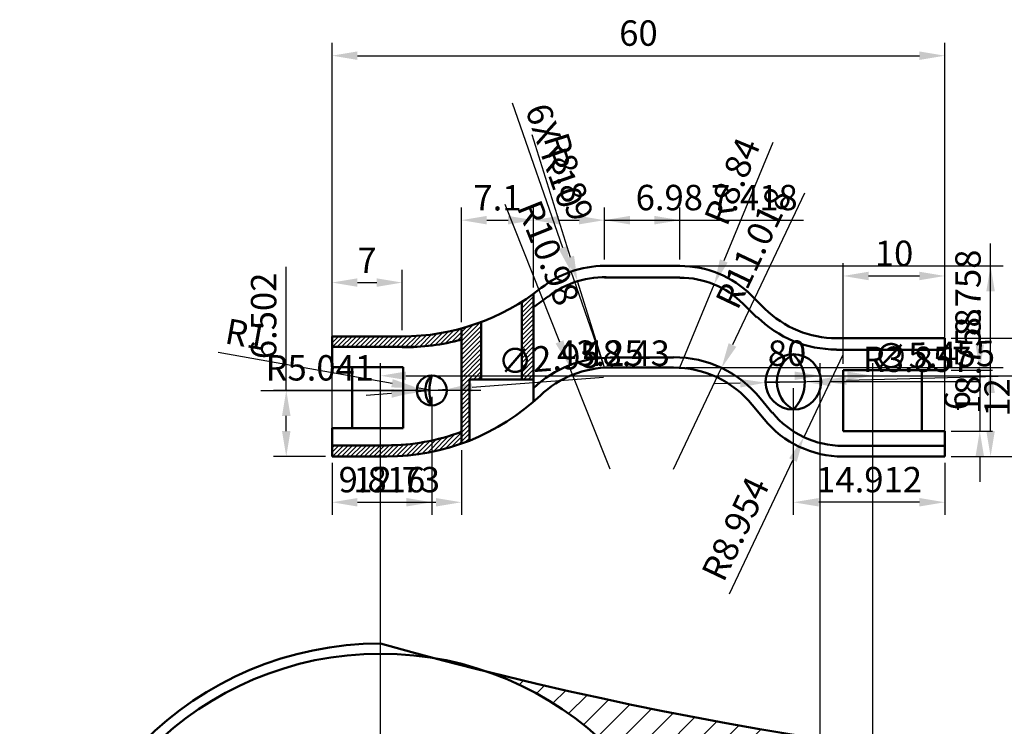
# Model space of a CAD drawing. Units: millimetres. Extents: x 1605 to 2079, y 1280 to 1879.
# Tile 3 of 7: x 1648 to 1745, y 1514 to 1583. Entities that reach past the tile are written whole.
import ezdxf

# ---------------------------------------------------------------- set-up
doc = ezdxf.new("R2010")
doc.units = ezdxf.units.MM
doc.linetypes.add('CENTER2', pattern=[28.574999999999996, 19.05, -3.174999999999999, 3.174999999999999, -3.174999999999999])
for name, color, linetype, lineweight in [('M-CNTR', 1, 'CENTER2', 18), ('M-DIMS', 2, 'Continuous', 25), ('M-HATC', 8, 'Continuous', 18), ('M-OUTL', 7, 'Continuous', 50)]:
    doc.layers.add(name, color=color, linetype=linetype, lineweight=lineweight)
doc.styles.get("Standard").update_dxf_attribs({"font": 'arial.ttf'})
doc.dimstyles.new('ISO-25', dxfattribs={"dimtxt": 2.5, "dimasz": 2.5, "dimexe": 1.25, "dimexo": 0.625, "dimtad": 1, "dimdec": 0, "dimtxsty": 'Standard', "dimcen": 2.5, "dimadec": 0, "dimazin": 0, "dimtfac": 1, "dimtdec": 0, "dimtmove": 0, "dimatfit": 3, "dimfxl": 1, "dimarcsym": 0})
pattern_1 = [(45, (0, 0), (-0.2245064030267288, 0.2245064030267288), [])]

# ---------------------------------------------------------------- blocks, each defined once
blk = doc.blocks.new('*U2')
at = {"layer": 'M-CNTR', "color": 0, "transparency": 16777216}
for p, q in [((0, 6.4), (0, 35.5)), ((-35.5, 0), (-6.399999999999998, 0)), ((6.4, 0), (35.5, 0)), ((0, -35.5), (0, -6.399999999999998))]:
    blk.add_line(p, q, dxfattribs=at)
at = {"layer": 'M-CNTR', "color": 0, "linetype": 'Continuous', "transparency": 16777216}
for p, q in [((0, -3.2), (0, 3.2)), ((-3.2, 0), (3.2, 0))]:
    blk.add_line(p, q, dxfattribs=at)
blk = doc.blocks.new('*D6')
at = {"layer": 'Defpoints', "color": 0, "transparency": 16777216}
for p in [(1738.945829042659, 1579.826881590476), (1678.645044474844, 1540.384347719754), (1738.945829042659, 1540.384347719754)]:
    blk.add_point(p, dxfattribs=at)
at = {"layer": 'M-DIMS', "color": 0, "lineweight": -2, "transparency": 16777216}
for p, q in [((1678.645044474844, 1541.009347719754), (1678.645044474844, 1581.076881590476)), ((1738.945829042659, 1541.009347719754), (1738.945829042659, 1581.076881590476)), ((1681.145044474844, 1579.826881590476), (1736.445829042659, 1579.826881590476))]:
    blk.add_line(p, q, dxfattribs=at)
at = {"layer": 'M-DIMS', "color": 0, "transparency": 16777216}
for points in [[(1681.145044474844, 1580.243548257142), (1681.145044474844, 1579.410214923809), (1678.645044474844, 1579.826881590476)], [(1736.445829042659, 1580.243548257142), (1736.445829042659, 1579.410214923809), (1738.945829042659, 1579.826881590476)]]:
    blk.add_solid(points, dxfattribs=at)
at = {"layer": 'M-DIMS', "color": 0, "transparency": 16777216, "insert": (1708.795436758752, 1581.72831405978), "char_height": 2.5, "attachment_point": 5}
blk.add_mtext('60', dxfattribs=at)
blk = doc.blocks.new('*D7')
at = {"layer": 'Defpoints', "color": 0, "transparency": 16777216}
for p in [(1685.55133154725, 1557.502449097515), (1678.645044474844, 1552.199565545558), (1685.55133154725, 1552.199565545558)]:
    blk.add_point(p, dxfattribs=at)
at = {"layer": 'M-DIMS', "color": 0, "lineweight": -2, "transparency": 16777216}
for p, q in [((1678.645044474844, 1552.824565545557), (1678.645044474844, 1558.752449097515)), ((1685.55133154725, 1552.824565545557), (1685.55133154725, 1558.752449097515)), ((1681.145044474844, 1557.502449097515), (1683.05133154725, 1557.502449097515))]:
    blk.add_line(p, q, dxfattribs=at)
at = {"layer": 'M-DIMS', "color": 0, "transparency": 16777216}
for points in [[(1681.145044474844, 1557.919115764181), (1681.145044474844, 1557.085782430848), (1678.645044474844, 1557.502449097515)], [(1683.05133154725, 1557.919115764181), (1683.05133154725, 1557.085782430848), (1685.55133154725, 1557.502449097515)]]:
    blk.add_solid(points, dxfattribs=at)
at = {"layer": 'M-DIMS', "color": 0, "transparency": 16777216, "insert": (1682.098188011047, 1559.377449097515), "char_height": 2.5, "attachment_point": 5}
blk.add_mtext('7', dxfattribs=at)
blk = doc.blocks.new('*D8')
at = {"layer": 'Defpoints', "color": 0, "transparency": 16777216}
for p in [(1738.94582904266, 1552.020572380303), (1738.94582904266, 1540.384347719755), (1746.290883843988, 1540.384347719755)]:
    blk.add_point(p, dxfattribs=at)
at = {"layer": 'M-DIMS', "color": 0, "lineweight": -2, "transparency": 16777216}
for p, q in [((1739.57082904266, 1552.020572380303), (1747.540883843988, 1552.020572380303)), ((1746.290883843988, 1549.520572380303), (1746.290883843988, 1542.884347719755)), ((1739.57082904266, 1540.384347719755), (1747.540883843988, 1540.384347719755))]:
    blk.add_line(p, q, dxfattribs=at)
at = {"layer": 'M-DIMS', "color": 0, "transparency": 16777216}
for points in [[(1745.874217177321, 1549.520572380303), (1746.707550510654, 1549.520572380303), (1746.290883843988, 1552.020572380303)], [(1745.874217177321, 1542.884347719755), (1746.707550510654, 1542.884347719755), (1746.290883843988, 1540.384347719755)]]:
    blk.add_solid(points, dxfattribs=at)
at = {"layer": 'M-DIMS', "color": 0, "transparency": 16777216, "insert": (1744.410767882187, 1546.202460050028), "char_height": 2.5, "attachment_point": 5, "rotation": 90}
blk.add_mtext('12', dxfattribs=at)
blk = doc.blocks.new('*D9')
at = {"layer": 'Defpoints', "color": 0, "transparency": 16777216}
for p in [(1738.94582904266, 1548.883072039406), (1738.94582904266, 1542.883072039406), (1742.3810871375, 1542.883072039406)]:
    blk.add_point(p, dxfattribs=at)
at = {"layer": 'M-DIMS', "color": 0, "lineweight": -2, "transparency": 16777216}
for p, q in [((1742.3810871375, 1551.383072039406), (1742.3810871375, 1553.883072039406)), ((1739.57082904266, 1548.883072039406), (1743.6310871375, 1548.883072039406)), ((1742.3810871375, 1548.883072039406), (1742.3810871375, 1542.883072039406)), ((1739.57082904266, 1542.883072039406), (1743.6310871375, 1542.883072039406)), ((1742.3810871375, 1540.383072039406), (1742.3810871375, 1537.883072039406))]:
    blk.add_line(p, q, dxfattribs=at)
at = {"layer": 'M-DIMS', "color": 0, "transparency": 16777216}
for points in [[(1741.964420470833, 1551.383072039406), (1742.797753804167, 1551.383072039406), (1742.3810871375, 1548.883072039406)], [(1741.964420470833, 1540.383072039406), (1742.797753804167, 1540.383072039406), (1742.3810871375, 1542.883072039406)]]:
    blk.add_solid(points, dxfattribs=at)
at = {"layer": 'M-DIMS', "color": 0, "transparency": 16777216, "insert": (1740.479654668195, 1545.883072039405), "char_height": 2.5, "attachment_point": 5, "rotation": 90}
blk.add_mtext('6', dxfattribs=at)
blk = doc.blocks.new('*D10')
at = {"layer": 'Defpoints', "color": 0, "transparency": 16777216}
for p in [(1738.945829042659, 1558.149744778363), (1728.945829042659, 1548.883072039405), (1738.945829042659, 1548.883072039405)]:
    blk.add_point(p, dxfattribs=at)
at = {"layer": 'M-DIMS', "color": 0, "lineweight": -2, "transparency": 16777216}
for p, q in [((1728.945829042659, 1549.508072039405), (1728.945829042659, 1559.399744778363)), ((1738.945829042659, 1549.508072039405), (1738.945829042659, 1559.399744778363)), ((1731.445829042659, 1558.149744778363), (1736.445829042659, 1558.149744778363))]:
    blk.add_line(p, q, dxfattribs=at)
at = {"layer": 'M-DIMS', "color": 0, "transparency": 16777216}
for points in [[(1731.445829042659, 1558.56641144503), (1731.445829042659, 1557.733078111696), (1728.945829042659, 1558.149744778363)], [(1736.445829042659, 1558.56641144503), (1736.445829042659, 1557.733078111696), (1738.945829042659, 1558.149744778363)]]:
    blk.add_solid(points, dxfattribs=at)
at = {"layer": 'M-DIMS', "color": 0, "transparency": 16777216, "insert": (1733.945829042659, 1560.051177247667), "char_height": 2.5, "attachment_point": 5}
blk.add_mtext('10', dxfattribs=at)
blk = doc.blocks.new('*D11')
at = {"layer": 'Defpoints', "color": 0, "transparency": 16777216}
for p in [(1687.009202827217, 1547.147898341788), (1688.460822472765, 1546.886649148962)]:
    blk.add_point(p, dxfattribs=at)
at = {"layer": 'M-DIMS', "color": 0, "lineweight": -2, "transparency": 16777216}
for p, q in [((1667.454793814781, 1550.667121566922), (1684.548732004864, 1547.590711318507)), ((1688.460822472765, 1546.886649148962), (1687.009202827217, 1547.147898341788))]:
    blk.add_line(p, q, dxfattribs=at)
at = {"layer": 'M-DIMS', "color": 0, "transparency": 16777216}
blk.add_solid([(1684.622534167651, 1548.000789788899), (1684.474929842078, 1547.180632848115), (1687.009202827217, 1547.147898341788)], dxfattribs=at)
at = {"layer": 'M-DIMS', "color": 0, "transparency": 16777216, "insert": (1670.149257494102, 1552.092518035817), "char_height": 2.5, "attachment_point": 5, "rotation": 349.79764513890115}
blk.add_mtext('R1', dxfattribs=at)
blk = doc.blocks.new('*D45')
at = {"layer": 'Defpoints', "color": 0, "transparency": 16777216}
for p in [(1763.415856, 1548.330601), (1683.415856, 1488.980601), (1763.415856, 1488.980601)]:
    blk.add_point(p, dxfattribs=at)
at = {"layer": 'M-DIMS', "color": 0, "lineweight": -2, "transparency": 16777216}
for p, q in [((1683.415856, 1489.605601), (1683.415856, 1549.580601)), ((1763.415856, 1489.605601), (1763.415856, 1549.580601)), ((1685.915856, 1548.330601), (1760.915856, 1548.330601))]:
    blk.add_line(p, q, dxfattribs=at)
at = {"layer": 'M-DIMS', "color": 0, "transparency": 16777216}
for points in [[(1685.915856, 1548.747267666666), (1685.915856, 1547.913934333333), (1683.415856, 1548.330601)], [(1760.915856, 1548.747267666666), (1760.915856, 1547.913934333333), (1763.415856, 1548.330601)]]:
    blk.add_solid(points, dxfattribs=at)
at = {"layer": 'M-DIMS', "color": 0, "transparency": 16777216, "insert": (1723.415856, 1550.232033469304), "char_height": 2.5, "attachment_point": 5}
blk.add_mtext('80', dxfattribs=at)
blk = doc.blocks.new('*D47')
at = {"layer": 'Defpoints', "color": 0, "transparency": 16777216}
for p in [(1726.666293, 1548.330601), (1683.415856, 1488.980601), (1726.666293, 1452.487829)]:
    blk.add_point(p, dxfattribs=at)
at = {"layer": 'M-DIMS', "color": 0, "lineweight": -2, "transparency": 16777216}
for p, q in [((1683.415856, 1489.605601), (1683.415856, 1549.580601)), ((1726.666293, 1453.112829), (1726.666293, 1549.580601)), ((1685.915856, 1548.330601), (1724.166293, 1548.330601))]:
    blk.add_line(p, q, dxfattribs=at)
at = {"layer": 'M-DIMS', "color": 0, "transparency": 16777216}
for points in [[(1685.915856, 1548.747267666666), (1685.915856, 1547.913934333333), (1683.415856, 1548.330601)], [(1724.166293, 1548.747267666666), (1724.166293, 1547.913934333333), (1726.666293, 1548.330601)]]:
    blk.add_solid(points, dxfattribs=at)
at = {"layer": 'M-DIMS', "color": 0, "transparency": 16777216, "insert": (1705.0410745, 1550.232886129604), "char_height": 2.5, "attachment_point": 5}
blk.add_mtext('43.25', dxfattribs=at)
blk = doc.blocks.new('*D49')
at = {"layer": 'Defpoints', "color": 0, "transparency": 16777216}
for p in [(1731.842463, 1548.330601), (1731.842463, 1511.839336), (1683.415856, 1488.980601)]:
    blk.add_point(p, dxfattribs=at)
at = {"layer": 'M-DIMS', "color": 0, "lineweight": -2, "transparency": 16777216}
for p, q in [((1683.415856, 1489.605601), (1683.415856, 1549.580601)), ((1731.842463, 1512.464336), (1731.842463, 1549.580601)), ((1685.915856, 1548.330601), (1729.342463, 1548.330601))]:
    blk.add_line(p, q, dxfattribs=at)
at = {"layer": 'M-DIMS', "color": 0, "transparency": 16777216}
for points in [[(1685.915856, 1548.747267666666), (1685.915856, 1547.913934333333), (1683.415856, 1548.330601)], [(1729.342463, 1548.747267666666), (1729.342463, 1547.913934333333), (1731.842463, 1548.330601)]]:
    blk.add_solid(points, dxfattribs=at)
at = {"layer": 'M-DIMS', "color": 0, "transparency": 16777216, "insert": (1707.6291595, 1550.232886129604), "char_height": 2.5, "attachment_point": 5}
blk.add_mtext('48.43', dxfattribs=at)
blk = doc.blocks.new('*D52')
at = {"layer": 'Defpoints', "color": 0, "transparency": 16777216}
for p in [(1712.872269000001, 1559.142254000001), (1743.445829000002, 1559.142254000001), (1738.945829000001, 1540.384348000001)]:
    blk.add_point(p, dxfattribs=at)
at = {"layer": 'M-DIMS', "color": 0, "lineweight": -2, "transparency": 16777216}
for p, q in [((1713.497269000001, 1559.142254000001), (1744.695829000002, 1559.142254000001)), ((1743.445829000002, 1542.884348000001), (1743.445829000002, 1556.642254000001)), ((1739.570829000001, 1540.384348000001), (1744.695829000002, 1540.384348000001))]:
    blk.add_line(p, q, dxfattribs=at)
at = {"layer": 'M-DIMS', "color": 0, "transparency": 16777216}
for points in [[(1743.029162333335, 1556.642254000001), (1743.862495666668, 1556.642254000001), (1743.445829000002, 1559.142254000001)], [(1743.029162333335, 1542.884348000001), (1743.862495666668, 1542.884348000001), (1743.445829000002, 1540.384348000001)]]:
    blk.add_solid(points, dxfattribs=at)
at = {"layer": 'M-DIMS', "color": 0, "transparency": 16777216, "insert": (1741.544396530698, 1549.763301), "char_height": 2.5, "attachment_point": 5, "rotation": 90}
blk.add_mtext('18.758', dxfattribs=at)
blk = doc.blocks.new('*D53')
at = {"layer": 'Defpoints', "color": 0, "transparency": 16777216}
for p in [(1691.374813, 1541.647874), (1678.645044, 1540.384348), (1691.374813, 1535.884348)]:
    blk.add_point(p, dxfattribs=at)
at = {"layer": 'M-DIMS', "color": 0, "lineweight": -2, "transparency": 16777216}
for p, q in [((1691.374813, 1541.022874), (1691.374813, 1534.634348)), ((1678.645044, 1539.759348), (1678.645044, 1534.634348)), ((1681.145044, 1535.884348), (1688.874813, 1535.884348))]:
    blk.add_line(p, q, dxfattribs=at)
at = {"layer": 'M-DIMS', "color": 0, "transparency": 16777216}
for points in [[(1681.145044, 1536.301014666667), (1681.145044, 1535.467681333333), (1678.645044, 1535.884348)], [(1688.874813, 1536.301014666667), (1688.874813, 1535.467681333333), (1691.374813, 1535.884348)]]:
    blk.add_solid(points, dxfattribs=at)
at = {"layer": 'M-DIMS', "color": 0, "transparency": 16777216, "insert": (1685.0099285, 1537.786633129604), "char_height": 2.5, "attachment_point": 5}
blk.add_mtext('12.73', dxfattribs=at)
blk = doc.blocks.new('*D54')
at = {"layer": 'Defpoints', "color": 0, "transparency": 16777216}
for p in [(1698.474129, 1563.642254), (1698.474129, 1556.395035), (1691.374813, 1552.98431)]:
    blk.add_point(p, dxfattribs=at)
at = {"layer": 'M-DIMS', "color": 0, "lineweight": -2, "transparency": 16777216}
for p, q in [((1691.374813, 1553.60931), (1691.374813, 1564.892254)), ((1698.474129, 1557.020035), (1698.474129, 1564.892254)), ((1693.874813, 1563.642254), (1695.974129, 1563.642254))]:
    blk.add_line(p, q, dxfattribs=at)
at = {"layer": 'M-DIMS', "color": 0, "transparency": 16777216}
for points in [[(1693.874813, 1564.058920666667), (1693.874813, 1563.225587333333), (1691.374813, 1563.642254)], [(1695.974129, 1564.058920666667), (1695.974129, 1563.225587333333), (1698.474129, 1563.642254)]]:
    blk.add_solid(points, dxfattribs=at)
at = {"layer": 'M-DIMS', "color": 0, "transparency": 16777216, "insert": (1694.924471, 1565.522369961801), "char_height": 2.5, "attachment_point": 5}
blk.add_mtext('7.1', dxfattribs=at)
blk = doc.blocks.new('*D55')
at = {"layer": 'Defpoints', "color": 0, "transparency": 16777216}
for p in [(1705.454375, 1563.642254), (1705.454375, 1559.142254), (1698.474129, 1556.395035)]:
    blk.add_point(p, dxfattribs=at)
at = {"layer": 'M-DIMS', "color": 0, "lineweight": -2, "transparency": 16777216}
for p, q in [((1698.474129, 1557.020035), (1698.474129, 1564.892254)), ((1705.454375, 1559.767254), (1705.454375, 1564.892254)), ((1700.974129, 1563.642254), (1702.954375, 1563.642254)), ((1705.454375, 1563.642254), (1715.716994372442, 1563.642254))]:
    blk.add_line(p, q, dxfattribs=at)
at = {"layer": 'M-DIMS', "color": 0, "transparency": 16777216}
for points in [[(1700.974129, 1564.058920666667), (1700.974129, 1563.225587333333), (1698.474129, 1563.642254)], [(1702.954375, 1564.058920666667), (1702.954375, 1563.225587333333), (1705.454375, 1563.642254)]]:
    blk.add_solid(points, dxfattribs=at)
at = {"layer": 'M-DIMS', "color": 0, "transparency": 16777216, "insert": (1711.835684686221, 1565.543686469304), "char_height": 2.5, "attachment_point": 5}
blk.add_mtext('6.98', dxfattribs=at)
blk = doc.blocks.new('*D56')
at = {"layer": 'Defpoints', "color": 0, "transparency": 16777216}
for p in [(1712.872269, 1563.642254), (1705.454375, 1559.142254), (1712.872269, 1559.142254)]:
    blk.add_point(p, dxfattribs=at)
at = {"layer": 'M-DIMS', "color": 0, "lineweight": -2, "transparency": 16777216}
for p, q in [((1705.454375, 1559.767254), (1705.454375, 1564.892254)), ((1712.872269, 1559.767254), (1712.872269, 1564.892254)), ((1707.954375, 1563.642254), (1710.372269, 1563.642254)), ((1712.872269, 1563.642254), (1725.043142124147, 1563.642254))]:
    blk.add_line(p, q, dxfattribs=at)
at = {"layer": 'M-DIMS', "color": 0, "transparency": 16777216}
for points in [[(1707.954375, 1564.058920666667), (1707.954375, 1563.225587333333), (1705.454375, 1563.642254)], [(1710.372269, 1564.058920666667), (1710.372269, 1563.225587333333), (1712.872269, 1563.642254)]]:
    blk.add_solid(points, dxfattribs=at)
at = {"layer": 'M-DIMS', "color": 0, "transparency": 16777216, "insert": (1720.207705562074, 1565.543686469304), "char_height": 2.5, "attachment_point": 5}
blk.add_mtext('7.418', dxfattribs=at)
blk = doc.blocks.new('*D57')
at = {"layer": 'Defpoints', "color": 0, "transparency": 16777216}
for p in [(1688.460822, 1546.886649), (1678.645044, 1540.384348), (1688.460822, 1535.884348)]:
    blk.add_point(p, dxfattribs=at)
at = {"layer": 'M-DIMS', "color": 0, "lineweight": -2, "transparency": 16777216}
for p, q in [((1688.460822, 1546.261649), (1688.460822, 1534.634348)), ((1678.645044, 1539.759348), (1678.645044, 1534.634348)), ((1681.145044, 1535.884348), (1685.960822, 1535.884348))]:
    blk.add_line(p, q, dxfattribs=at)
at = {"layer": 'M-DIMS', "color": 0, "transparency": 16777216}
for points in [[(1681.145044, 1536.301014666667), (1681.145044, 1535.467681333333), (1678.645044, 1535.884348)], [(1685.960822, 1536.301014666667), (1685.960822, 1535.467681333333), (1688.460822, 1535.884348)]]:
    blk.add_solid(points, dxfattribs=at)
at = {"layer": 'M-DIMS', "color": 0, "transparency": 16777216, "insert": (1683.552933, 1537.785780469304), "char_height": 2.5, "attachment_point": 5}
blk.add_mtext('9.816', dxfattribs=at)
blk = doc.blocks.new('*D58')
at = {"layer": 'Defpoints', "color": 0, "transparency": 16777216}
for p in [(1674.145044000002, 1546.886649000001), (1688.460822000001, 1546.886649000001), (1678.645044000001, 1540.384348000001)]:
    blk.add_point(p, dxfattribs=at)
at = {"layer": 'M-DIMS', "color": 0, "lineweight": -2, "transparency": 16777216}
for p, q in [((1674.145044000002, 1546.886649000001), (1674.145044000002, 1559.060932765349)), ((1687.835822000001, 1546.886649000001), (1672.895044000002, 1546.886649000001)), ((1674.145044000002, 1542.884348000001), (1674.145044000002, 1544.386649000001)), ((1678.020044000001, 1540.384348000001), (1672.895044000002, 1540.384348000001))]:
    blk.add_line(p, q, dxfattribs=at)
at = {"layer": 'M-DIMS', "color": 0, "transparency": 16777216}
for points in [[(1673.728377333335, 1544.386649000001), (1674.561710666668, 1544.386649000001), (1674.145044000002, 1546.886649000001)], [(1673.728377333335, 1542.884348000001), (1674.561710666668, 1542.884348000001), (1674.145044000002, 1540.384348000001)]]:
    blk.add_solid(points, dxfattribs=at)
at = {"layer": 'M-DIMS', "color": 0, "transparency": 16777216, "insert": (1672.243611530698, 1554.223790882674), "char_height": 2.5, "attachment_point": 5, "rotation": 90}
blk.add_mtext('6.502', dxfattribs=at)
blk = doc.blocks.new('*D59')
at = {"layer": 'Defpoints', "color": 0, "transparency": 16777216}
for p in [(1724.033427, 1547.729634), (1738.945829, 1540.384348), (1724.033427, 1535.884348)]:
    blk.add_point(p, dxfattribs=at)
at = {"layer": 'M-DIMS', "color": 0, "lineweight": -2, "transparency": 16777216}
for p, q in [((1724.033427, 1547.104634), (1724.033427, 1534.634348)), ((1738.945829, 1539.759348), (1738.945829, 1534.634348)), ((1736.445829, 1535.884348), (1726.533427, 1535.884348))]:
    blk.add_line(p, q, dxfattribs=at)
at = {"layer": 'M-DIMS', "color": 0, "transparency": 16777216}
for points in [[(1726.533427, 1536.301014666667), (1726.533427, 1535.467681333333), (1724.033427, 1535.884348)], [(1736.445829, 1536.301014666667), (1736.445829, 1535.467681333333), (1738.945829, 1535.884348)]]:
    blk.add_solid(points, dxfattribs=at)
at = {"layer": 'M-DIMS', "color": 0, "transparency": 16777216, "insert": (1731.489628, 1537.785780469304), "char_height": 2.5, "attachment_point": 5}
blk.add_mtext('14.912', dxfattribs=at)
blk = doc.blocks.new('*D60')
at = {"layer": 'Defpoints', "color": 0, "transparency": 16777216}
for p in [(1712.872269000001, 1549.142254000001), (1743.445829000002, 1549.142254000001), (1738.945829000001, 1540.384348000001)]:
    blk.add_point(p, dxfattribs=at)
at = {"layer": 'M-DIMS', "color": 0, "lineweight": -2, "transparency": 16777216}
for p, q in [((1743.445829000002, 1549.142254000001), (1743.445829000002, 1561.337001612552)), ((1713.497269000001, 1549.142254000001), (1744.695829000002, 1549.142254000001)), ((1743.445829000002, 1542.884348000001), (1743.445829000002, 1546.642254000001)), ((1739.570829000001, 1540.384348000001), (1744.695829000002, 1540.384348000001))]:
    blk.add_line(p, q, dxfattribs=at)
at = {"layer": 'M-DIMS', "color": 0, "transparency": 16777216}
for points in [[(1743.029162333335, 1546.642254000001), (1743.862495666668, 1546.642254000001), (1743.445829000002, 1549.142254000001)], [(1743.029162333335, 1542.884348000001), (1743.862495666668, 1542.884348000001), (1743.445829000002, 1540.384348000001)]]:
    blk.add_solid(points, dxfattribs=at)
at = {"layer": 'M-DIMS', "color": 0, "transparency": 16777216, "insert": (1741.544396530698, 1556.489627806275), "char_height": 2.5, "attachment_point": 5, "rotation": 90}
blk.add_mtext('8.758', dxfattribs=at)
blk = doc.blocks.new('*D73')
at = {"layer": 'Defpoints', "color": 0, "transparency": 16777216}
for p in [(1702.160883, 1558.584336), (1705.454374999999, 1549.142254)]:
    blk.add_point(p, dxfattribs=at)
at = {"layer": 'M-DIMS', "color": 0, "lineweight": -2, "transparency": 16777216}
for p, q in [((1696.36413494683, 1575.202979813729), (1701.337510008434, 1560.944856475819)), ((1705.454374999999, 1549.142254), (1702.160883, 1558.584336))]:
    blk.add_line(p, q, dxfattribs=at)
at = {"layer": 'M-DIMS', "color": 0, "transparency": 16777216}
blk.add_solid([(1701.730930087737, 1561.082085307746), (1700.944089929131, 1560.807627643891), (1702.160883, 1558.584336)], dxfattribs=at)
at = {"layer": 'M-DIMS', "color": 0, "transparency": 16777216, "insert": (1700.234484092722, 1569.880413638887), "char_height": 2.5, "attachment_point": 5, "rotation": 289.22927914580976}
blk.add_mtext('6X R10', dxfattribs=at)
blk = doc.blocks.new('*D74')
at = {"layer": 'Defpoints', "color": 0, "transparency": 16777216}
for p in [(1716.975232, 1549.099488999999), (1712.257654, 1539.142253999999)]:
    blk.add_point(p, dxfattribs=at)
at = {"layer": 'M-DIMS', "color": 0, "lineweight": -2, "transparency": 16777216}
for p, q in [((1725.12151537231, 1566.293578406614), (1718.045631876652, 1551.358746423151)), ((1712.257654, 1539.142253999999), (1716.975232, 1549.099488999999))]:
    blk.add_line(p, q, dxfattribs=at)
at = {"layer": 'M-DIMS', "color": 0, "transparency": 16777216}
blk.add_solid([(1717.669088972794, 1551.537146402593), (1718.422174780511, 1551.180346443709), (1716.975232, 1549.099488999999)], dxfattribs=at)
at = {"layer": 'M-DIMS', "color": 0, "transparency": 16777216, "insert": (1720.400443394449, 1560.7699083587), "char_height": 2.5, "attachment_point": 5, "rotation": 64.64915745028115}
blk.add_mtext('R11.018', dxfattribs=at)
blk = doc.blocks.new('*D75')
at = {"layer": 'Defpoints', "color": 0, "transparency": 16777216}
for p in [(1701.959906999999, 1549.344234999999), (1706.022004999999, 1539.142254)]:
    blk.add_point(p, dxfattribs=at)
at = {"layer": 'M-DIMS', "color": 0, "lineweight": -2, "transparency": 16777216}
for p, q in [((1695.640185789668, 1565.21624884927), (1701.035100522225, 1551.666891448695)), ((1706.022004999999, 1539.142254), (1701.959906999999, 1549.344234999999))]:
    blk.add_line(p, q, dxfattribs=at)
at = {"layer": 'M-DIMS', "color": 0, "transparency": 16777216}
blk.add_solid([(1701.42220993034, 1551.821025861657), (1700.647991114109, 1551.512757035732), (1701.959906999999, 1549.344234999999)], dxfattribs=at)
at = {"layer": 'M-DIMS', "color": 0, "transparency": 16777216, "insert": (1699.641789671695, 1560.306281199195), "char_height": 2.5, "attachment_point": 5, "rotation": 291.71084335696685}
blk.add_mtext('R10.98', dxfattribs=at)
blk = doc.blocks.new('*D76')
at = {"layer": 'Defpoints', "color": 0, "transparency": 16777216}
for p in [(1728.901096, 1550.384348), (1725.067011, 1542.293023)]:
    blk.add_point(p, dxfattribs=at)
at = {"layer": 'M-DIMS', "color": 0, "lineweight": -2, "transparency": 16777216}
for p, q in [((1728.901096, 1550.384348), (1725.067011, 1542.293023)), ((1717.758091055393, 1526.868522324926), (1723.996486807893, 1540.033824479702))]:
    blk.add_line(p, q, dxfattribs=at)
at = {"layer": 'M-DIMS', "color": 0, "transparency": 16777216}
blk.add_solid([(1723.619953721177, 1540.212245178387), (1724.373019894609, 1539.855403781018), (1725.067011, 1542.293023)], dxfattribs=at)
at = {"layer": 'M-DIMS', "color": 0, "transparency": 16777216, "insert": (1718.623741467151, 1533.135785925383), "char_height": 2.5, "attachment_point": 5, "rotation": 64.64600471361501}
blk.add_mtext('R8.954', dxfattribs=at)
blk = doc.blocks.new('*D77')
at = {"layer": 'Defpoints', "color": 0, "transparency": 16777216}
for p in [(1702.806965, 1557.629112999999), (1705.454374999999, 1549.142253999999)]:
    blk.add_point(p, dxfattribs=at)
at = {"layer": 'M-DIMS', "color": 0, "lineweight": -2, "transparency": 16777216}
for p, q in [((1698.297966980106, 1572.083704629602), (1702.062490273435, 1560.015691593196)), ((1705.454374999999, 1549.142253999999), (1702.806965, 1557.629112999999))]:
    blk.add_line(p, q, dxfattribs=at)
at = {"layer": 'M-DIMS', "color": 0, "transparency": 16777216}
blk.add_solid([(1702.460253372301, 1560.13977071429), (1701.664727174569, 1559.891612472102), (1702.806965, 1557.629112999999)], dxfattribs=at)
at = {"layer": 'M-DIMS', "color": 0, "transparency": 16777216, "insert": (1701.623158474549, 1567.809214775064), "char_height": 2.5, "attachment_point": 5, "rotation": 287.32490708382795}
blk.add_mtext('R8.89', dxfattribs=at)
blk = doc.blocks.new('*D78')
at = {"layer": 'Defpoints', "color": 0, "transparency": 16777216}
for p in [(1716.242073, 1557.315176), (1712.872269, 1549.142254)]:
    blk.add_point(p, dxfattribs=at)
at = {"layer": 'M-DIMS', "color": 0, "lineweight": -2, "transparency": 16777216}
for p, q in [((1722.007926505024, 1571.299333820451), (1717.195031425971, 1559.62642463188)), ((1712.872269, 1549.142254), (1716.242073, 1557.315176))]:
    blk.add_line(p, q, dxfattribs=at)
at = {"layer": 'M-DIMS', "color": 0, "transparency": 16777216}
blk.add_solid([(1716.809823320658, 1559.785251036209), (1717.580239531285, 1559.467598227552), (1716.242073, 1557.315176)], dxfattribs=at)
at = {"layer": 'M-DIMS', "color": 0, "transparency": 16777216, "insert": (1718.320084901166, 1567.343297979322), "char_height": 2.5, "attachment_point": 5, "rotation": 67.59299737995454}
blk.add_mtext('R8.84', dxfattribs=at)
blk = doc.blocks.new('*D79')
at = {"layer": 'Defpoints', "color": 0, "transparency": 16777216}
for p in [(1688.240238, 1546.887), (1693.281636, 1546.886649)]:
    blk.add_point(p, dxfattribs=at)
at = {"layer": 'M-DIMS', "color": 0, "lineweight": -2, "transparency": 16777216}
for p, q in [((1671.64405795837, 1546.888155484886), (1685.74023800606, 1546.887174058862)), ((1693.281636, 1546.886649), (1688.240238, 1546.887))]:
    blk.add_line(p, q, dxfattribs=at)
at = {"layer": 'M-DIMS', "color": 0, "transparency": 16777216}
blk.add_solid([(1685.74026701587, 1547.303840724518), (1685.740208996249, 1546.470507393205), (1688.240238, 1546.887)], dxfattribs=at)
at = {"layer": 'M-DIMS', "color": 0, "transparency": 16777216, "insert": (1677.442280369713, 1548.789184266), "char_height": 2.5, "attachment_point": 5, "rotation": 359.9960108647301}
blk.add_mtext('R5.041', dxfattribs=at)
blk = doc.blocks.new('*D80')
at = {"layer": 'Defpoints', "color": 0, "transparency": 16777216}
for p in [(1721.305945999999, 1547.729633999999), (1725.163186999999, 1547.729999999999)]:
    blk.add_point(p, dxfattribs=at)
at = {"layer": 'M-DIMS', "color": 0, "lineweight": -2, "transparency": 16777216}
for p, q in [((1721.305945999999, 1547.729633999999), (1725.163186999999, 1547.729999999999)), ((1742.241972734849, 1547.731620545767), (1727.663186988745, 1547.730237216185))]:
    blk.add_line(p, q, dxfattribs=at)
at = {"layer": 'M-DIMS', "color": 0, "transparency": 16777216}
blk.add_solid([(1727.663147452714, 1548.146903880976), (1727.663226524776, 1547.313570551394), (1725.163186999999, 1547.729999999999)], dxfattribs=at)
at = {"layer": 'M-DIMS', "color": 0, "transparency": 16777216, "insert": (1736.202399355041, 1549.63333261011), "char_height": 2.5, "attachment_point": 5, "rotation": 0.0054365945083347765}
blk.add_mtext('R3.857', dxfattribs=at)
blk = doc.blocks.new('*D81')
at = {"layer": 'Defpoints', "color": 0, "transparency": 16777216}
for p in [(1686.990023, 1546.776181), (1689.931621, 1546.997117)]:
    blk.add_point(p, dxfattribs=at)
at = {"layer": 'M-DIMS', "color": 0, "lineweight": -2, "transparency": 16777216}
for p, q in [((1705.370740907403, 1548.156710321676), (1692.424599277812, 1547.184358305163)), ((1684.497044722188, 1546.588939694837), (1682.004066444377, 1546.401698389674)), ((1686.990023, 1546.776181), (1689.931621, 1546.997117))]:
    blk.add_line(p, q, dxfattribs=at)
at = {"layer": 'M-DIMS', "color": 0, "transparency": 16777216}
for points in [[(1692.393392393618, 1547.599854684798), (1692.455806162006, 1546.768861925527), (1689.931621, 1546.997117)], [(1684.465837837994, 1547.004436074472), (1684.528251606382, 1546.173443315202), (1686.990023, 1546.776181)]]:
    blk.add_solid(points, dxfattribs=at)
at = {"layer": 'M-DIMS', "color": 0, "transparency": 16777216, "insert": (1699.996511926759, 1549.729968669378), "char_height": 2.5, "attachment_point": 5, "rotation": 4.295276733366178}
blk.add_mtext('∅2.95', dxfattribs=at)
blk = doc.blocks.new('*D82')
at = {"layer": 'Defpoints', "color": 0, "transparency": 16777216}
for p in [(1721.306873, 1547.658486), (1726.759981, 1547.800782)]:
    blk.add_point(p, dxfattribs=at)
at = {"layer": 'M-DIMS', "color": 0, "lineweight": -2, "transparency": 16777216}
for p, q in [((1744.179017402703, 1548.255322640669), (1729.259130282283, 1547.865995992877)), ((1718.807723717718, 1547.593272007122), (1716.308574435435, 1547.528058014245)), ((1721.306873, 1547.658486), (1726.759981, 1547.800782))]:
    blk.add_line(p, q, dxfattribs=at)
at = {"layer": 'M-DIMS', "color": 0, "transparency": 16777216}
for points in [[(1729.248261283469, 1548.282520873258), (1729.269999281095, 1547.449471112497), (1726.759981, 1547.800782)], [(1718.796854718904, 1548.009796887503), (1718.81859271653, 1547.176747126742), (1721.306873, 1547.658486)]]:
    blk.add_solid(points, dxfattribs=at)
at = {"layer": 'M-DIMS', "color": 0, "transparency": 16777216, "insert": (1737.917224625676, 1550.06394610197), "char_height": 2.5, "attachment_point": 5, "rotation": 1.494764176324067}
blk.add_mtext('∅5.455', dxfattribs=at)

msp = doc.modelspace()

# ---------------------------------------------------------------- hatches: boundary and pattern name
at = {"layer": 'M-HATC'}
h = msp.add_hatch(dxfattribs=at)
h.set_pattern_fill('ANSI31', color=256, scale=0.1)
h.set_pattern_definition(pattern_1)
h.paths.add_polyline_path([(1698.474128719783, 1556.395034851446, -0.0158606141869828), (1697.319423953205, 1555.611612427344), (1697.319423953205, 1547.976652959475), (1698.474128719783, 1547.976652959475)])
h = msp.add_hatch(dxfattribs=at)
h.set_pattern_fill('ANSI31', color=256, scale=0.1)
h.set_pattern_definition(pattern_1)
h.paths.add_polyline_path([(1693.319423953205, 1553.616642031816, -0.0232493374510837), (1691.374812892836, 1552.984310067067), (1691.374812892836, 1541.647873975909, 0.0095909802093284), (1692.164719186626, 1541.944965840922), (1692.164719186626, 1547.976652959475), (1693.319423953205, 1547.976652959475)])
h.paths.add_polyline_path([(1691.374812892836, 1541.647873975909), (1691.374812892836, 1542.817802922434, -0.0900572933523556), (1684.026435067029, 1541.483430706945), (1678.645044474844, 1541.483430706945), (1678.645044474844, 1540.384347719754), (1684.026435067029, 1540.384347719754, 0.0853469052335504)])
h.paths.add_polyline_path([(1691.374812892836, 1551.877660089471), (1691.374812892836, 1552.984310067067, -0.0670744800772869), (1685.551331547249, 1552.199565545558), (1678.645044474844, 1552.199565545558), (1678.645044474844, 1551.171994767597), (1686.933859029395, 1551.171994767597, 0.0488468451239397)])
h = msp.add_hatch(dxfattribs=at)
h.set_pattern_fill('ANSI31', color=256, scale=0.5700000000000001)
h.set_pattern_definition([(45, (0, 0), (-1.279686497252354, 1.279686497252354), [])])
edge = h.paths.add_edge_path()
edge.add_spline(control_points=[(1735.07459974606, 1431.314795075923), (1745.983278041014, 1442.572726331581), (1760.24984788448, 1457.296055612093), (1736.483989804082, 1465.949384402775), (1733.184296285201, 1487.573131299177), (1732.318614147286, 1503.228440483471), (1731.842462696298, 1511.83933570387)], knot_values=[0, 0, 0, 0, 32.3106591245444, 42.25647348148218, 64.0151754338639, 90.61240603446909, 90.61240603446909, 90.61240603446909, 90.61240603446909], degree=3, periodic=0)
edge.add_arc((1783.415855978972, 1878.806874192082), 370.5738647001252, 256.0328658121666, 262.00008128327465, ccw=False)
edge.add_arc((1683.415855978972, 1488.98060105796), 32, 0, 70.73817384477002, ccw=False)
edge.add_arc((1683.415855978972, 1488.98060105796), 32, -90, 0, ccw=False)
edge.add_line((1683.415855978972, 1456.98060105796), (1683.415855978972, 1455.98060105796))
edge.add_line((1683.415855978972, 1455.98060105796), (1735.07459974606, 1431.314795075923))
h.paths.add_polyline_path([(1726.66629323774, 1456.237829432783), (1741.66629323774, 1456.237829432783, -1), (1741.66629323774, 1448.737829432783), (1726.66629323774, 1448.737829432783, -1)], flags=16)
h.paths.add_polyline_path([(1731.47870797171, 1442.133012605171), (1736.613428299132, 1442.133012605171), (1736.613428299132, 1447.284786138595), (1731.47870797171, 1447.284786138595)], flags=24)
h.paths.add_polyline_path([(1713.173444990596, 1457.268825178529), (1718.453947385105, 1455.084302360538), (1720.423342620304, 1459.844791090414), (1715.142840225795, 1462.029313908404)], flags=24)

# ---------------------------------------------------------------- linework, layer by layer
at = {"layer": 'M-OUTL'}
for p, q in [((1705.454375346341, 1559.142254286537), (1712.872268745755, 1559.142254286537)), ((1705.454375346341, 1558.012835433478), (1712.872268745755, 1558.012835433478)), ((1698.474128719783, 1547.117880511772), (1698.474128719783, 1556.395034851446)), ((1719.920675000811, 1556.23591126046), (1721.238074599122, 1554.926915406378)), ((1697.319423953205, 1555.611612427344), (1697.319423953205, 1547.976652959475)), ((1719.090085348781, 1555.399989228672), (1720.407484947091, 1554.09099337459)), ((1691.374812892836, 1552.984310067067), (1691.374812892836, 1541.647873975909)), ((1693.319423953205, 1547.976652959475), (1693.319423953205, 1553.616642031816)), ((1678.645044474844, 1552.199565545558), (1685.55133154725, 1552.199565545558)), ((1678.645044474844, 1552.199565545558), (1678.645044474844, 1551.171994767597)), ((1728.286480854178, 1552.020572380302), (1738.945829042659, 1552.020572380302)), ((1738.945829042659, 1552.020572380302), (1738.945829042659, 1550.883072039405)), ((1678.645044474844, 1551.171994767597), (1686.933859029396, 1551.171994767597)), ((1678.645044474844, 1551.171994767597), (1678.645044474844, 1549.171994767597)), ((1706.022004912832, 1550.134855091574), (1712.25765375976, 1550.134855091574)), ((1728.286480854178, 1550.883072039405), (1738.945829042659, 1550.883072039405)), ((1738.945829042659, 1550.883072039405), (1738.945829042659, 1548.883072039405)), ((1678.645044474844, 1549.171994767597), (1685.645044474844, 1549.171994767597)), ((1680.636614060281, 1549.171994767597), (1680.63661406028, 1543.171994767597)), ((1685.645044474844, 1549.171994767597), (1685.645044474844, 1545.171994767597)), ((1706.022004912832, 1549.142254286536), (1712.25765375976, 1549.142254286536)), ((1738.945829042659, 1548.883072039405), (1728.945829042659, 1548.883072039405)), ((1728.945829042659, 1548.883072039405), (1728.945829042659, 1544.883072039405)), ((1736.680516214728, 1548.883072039405), (1736.680516214728, 1542.883072039405)), ((1692.164719186626, 1541.944965840922), (1692.164719186626, 1547.976652959475)), ((1692.164719186626, 1547.976652959475), (1698.474128719783, 1547.976652959475)), ((1695.319423953205, 1547.976652959475), (1693.319423953205, 1547.976652959475)), ((1698.474128719783, 1547.117880511772), (1698.474128719783, 1545.793261314212)), ((1719.996428487772, 1545.475607719678), (1721.162321112162, 1544.050994286612)), ((1720.784437397952, 1546.120508122138), (1721.950330022343, 1544.695894689072)), ((1685.645044474844, 1545.171994767597), (1685.645044474844, 1544.171994767597)), ((1728.945829042659, 1544.883072039405), (1728.945829042659, 1542.883072039405)), ((1685.645044474844, 1544.171994767597), (1685.645044474844, 1543.171994767597)), ((1681.645044474844, 1543.171994767597), (1678.645044474844, 1543.171994767597)), ((1678.645044474844, 1543.171994767597), (1678.645044474844, 1541.483430706945)), ((1685.645044474844, 1543.171994767597), (1681.645044474844, 1543.171994767597)), ((1728.945829042659, 1542.883072039405), (1738.945829042659, 1542.883072039405)), ((1738.945829042659, 1542.883072039405), (1738.945829042659, 1541.441282449549)), ((1678.645044474844, 1541.483430706945), (1684.026435067029, 1541.483430706945)), ((1678.645044474844, 1541.483430706945), (1678.645044474844, 1540.384347719754)), ((1728.901095840173, 1541.441282449549), (1738.945829042659, 1541.441282449549)), ((1738.945829042659, 1541.441282449549), (1738.945829042659, 1540.384347719754)), ((1678.645044474844, 1540.384347719754), (1684.026435067029, 1540.384347719754)), ((1728.901095840173, 1540.384347719754), (1738.945829042659, 1540.384347719754))]:
    msp.add_line(p, q, dxfattribs=at)
for centre, radius in [((1724.033427437432, 1547.729633627987), 2.727481313842424), ((1688.460822472767, 1546.886649148965), 1.474940926307681), ((1683.415855978972, 1488.98060105796), 32)]:
    msp.add_circle(centre, radius, dxfattribs=at)
for centre, radius, start, end in [((1705.454375346341, 1549.142254286537), 10, 90, 128.4601461444616), ((1712.872268745755, 1549.142254286536), 10, 45.18333013514169, 90), ((1705.454375346341, 1549.142254286537), 8.890193827309176, 86.19346029287718, 128.4601461444616), ((1712.872268745755, 1549.142254286536), 8.840375060270613, 45.18333013514169, 90), ((1685.55133154725, 1574.199565545557), 22, 270, 308.460146144462), ((1685.55133154725, 1574.199565545557), 23.06903548423432, 304.0682015065403, 308.460146144462), ((1728.286480854178, 1562.020572380302), 10, 225.1833301351417, 270), ((1728.286480854178, 1562.020572380302), 11.1079010127712, 225.1833301351417, 270), ((1685.55133154725, 1574.199565545557), 23.06903548423432, 270, 284.621776583433), ((1706.022004912832, 1539.142254286537), 10.98094024709417, 90, 133.4216144763459), ((1712.25765375976, 1539.142254286536), 11.01826056175077, 39.29662905253368, 90), ((1725.523062650189, 1547.729633627987), 3.10775922240486, 118.6415050293552, 241.3584949706419), ((1721.30594612359, 1547.729633627987), 3.857241065154974, 314.9999999999952, 45), ((1706.022004912832, 1539.142254286537), 10, 90, 133.4216144763459), ((1712.25765375976, 1539.142254286536), 10, 39.29662905253368, 90), ((1689.831735590376, 1546.886649148965), 2.013666683473275, 132.9065329178466, 227.0934670821507), ((1693.281636018545, 1546.886649148965), 5.041398018332984, 162.9883673170949, 197.0116326829047), ((1684.026435067029, 1562.384347719754), 22, 270, 313.4216144763454), ((1728.901095840173, 1550.384347719754), 8.953755626304364, 219.2966290525345, 270), ((1728.901095840173, 1550.384347719754), 10, 219.2966290525345, 270), ((1684.026435067029, 1562.384347719754), 20.90091701280926, 270, 290.5840833301981), ((1683.415855978972, 1488.98060105796), 33, 90, 270), ((1783.415855978972, 1878.806874192082), 370.5738647001254, 254.3445556403036, 285.6554443596963)]:
    msp.add_arc(centre, radius, start, end, dxfattribs=at)

# ---------------------------------------------------------------- block references
at = {"layer": 'M-CNTR'}
msp.add_blockref('*U2', (1683.415855978972, 1488.98060105796), dxfattribs=at)

# ---------------------------------------------------------------- dimensions: what is measured, and where the dimension line sits
at = {"layer": 'M-DIMS'}
for base, p1, p2, override, picture, middle in [((1738.945829042659, 1579.826881590476), (1678.645044474844, 1540.384347719754), (1738.945829042659, 1540.384347719754), {"dimclrd": 0, "dimclre": 0, "dimclrt": 0}, '*D6', (1708.795436758752, 1581.72831405978)), ((1698.474129, 1563.642254), (1691.374813, 1552.98431), (1698.474129, 1556.395035), {"dimdec": 1, "dimlfac": 1, "dimrnd": 0, "dimzin": 0, "dimdsep": 46, "dimlunit": 2}, '*D54', (1694.924471, 1565.522369961801)), ((1705.454375, 1563.642254), (1698.474129, 1556.395035), (1705.454375, 1559.142254), {"dimdec": 2, "dimlfac": 1, "dimrnd": 0, "dimzin": 0, "dimdsep": 46, "dimlunit": 2}, '*D55', (1711.835684686221, 1565.543686469304)), ((1712.872269, 1563.642254), (1705.454375, 1559.142254), (1712.872269, 1559.142254), {"dimdec": 3, "dimlfac": 1, "dimrnd": 0, "dimzin": 0, "dimdsep": 46, "dimlunit": 2}, '*D56', (1720.207705562074, 1565.543686469304)), ((1738.945829042659, 1558.149744778363), (1728.945829042659, 1548.883072039405), (1738.945829042659, 1548.883072039405), {"dimclrd": 0, "dimclre": 0, "dimclrt": 0}, '*D10', (1733.945829042659, 1560.051177247667)), ((1685.55133154725, 1557.502449097515), (1678.645044474844, 1552.199565545558), (1685.55133154725, 1552.199565545558), {"dimclrd": 0, "dimclre": 0, "dimclrt": 0}, '*D7', (1682.098188011047, 1559.377449097515)), ((1726.666293, 1548.330601), (1683.415856, 1488.980601), (1726.666293, 1452.487829), {"dimdec": 2, "dimlfac": 1, "dimrnd": 0, "dimzin": 0, "dimdsep": 46, "dimlunit": 2}, '*D47', (1705.0410745, 1550.232886129604)), ((1731.842463, 1548.330601), (1683.415856, 1488.980601), (1731.842463, 1511.839336), {"dimdec": 2, "dimlfac": 1, "dimrnd": 0, "dimzin": 0, "dimdsep": 46, "dimlunit": 2}, '*D49', (1707.6291595, 1550.232886129604)), ((1763.415856, 1548.330601), (1683.415856, 1488.980601), (1763.415856, 1488.980601), {"dimdec": 0, "dimlfac": 1, "dimrnd": 0, "dimzin": 0, "dimdsep": 46, "dimlunit": 2}, '*D45', (1723.415856, 1550.232033469304)), ((1724.033427, 1535.884348), (1738.945829, 1540.384348), (1724.033427, 1547.729634), {"dimdec": 3, "dimlfac": 1, "dimrnd": 0, "dimzin": 0, "dimdsep": 46, "dimlunit": 2}, '*D59', (1731.489628, 1537.785780469304)), ((1688.460822, 1535.884348), (1678.645044, 1540.384348), (1688.460822, 1546.886649), {"dimdec": 3, "dimlfac": 1, "dimrnd": 0, "dimzin": 0, "dimdsep": 46, "dimlunit": 2}, '*D57', (1683.552933, 1537.785780469304)), ((1691.374813, 1535.884348), (1678.645044, 1540.384348), (1691.374813, 1541.647874), {"dimdec": 2, "dimlfac": 1, "dimrnd": 0, "dimzin": 0, "dimdsep": 46, "dimlunit": 2}, '*D53', (1685.0099285, 1537.786633129604))]:
    dim = msp.add_linear_dim(base=base, p1=p1, p2=p2, dimstyle='ISO-25', override=override, dxfattribs=at)
    dim.commit()
    dim.dimension.update_dxf_attribs({"geometry": picture, "text_midpoint": middle})
dim = msp.add_radius_dim(center=(1705.454374999999, 1549.142254), mpoint=(1702.160883, 1558.584336), text='6X <>', dimstyle='ISO-25', override={"dimdec": 0, "dimlfac": 1, "dimrnd": 0, "dimzin": 0, "dimdsep": 46, "dimlunit": 2}, dxfattribs=at)
dim.commit()
dim.dimension.update_dxf_attribs({"geometry": '*D73', "text_midpoint": (1700.234484092722, 1569.880413638887)})
for center, mpoint, override, picture, middle in [((1705.454374999999, 1549.142253999999), (1702.806965, 1557.629112999999), {"dimdec": 2, "dimlfac": 1, "dimrnd": 0, "dimzin": 0, "dimdsep": 46, "dimlunit": 2}, '*D77', (1701.623158474549, 1567.809214775064)), ((1712.872269, 1549.142254), (1716.242073, 1557.315176), {"dimdec": 2, "dimlfac": 1, "dimrnd": 0, "dimzin": 0, "dimdsep": 46, "dimlunit": 2}, '*D78', (1718.320084901166, 1567.343297979322)), ((1712.257654, 1539.142253999999), (1716.975232, 1549.099488999999), {"dimdec": 3, "dimlfac": 1, "dimrnd": 0, "dimzin": 0, "dimdsep": 46, "dimlunit": 2}, '*D74', (1720.400443394449, 1560.7699083587)), ((1706.022004999999, 1539.142254), (1701.959906999999, 1549.344234999999), {"dimdec": 2, "dimlfac": 1, "dimrnd": 0, "dimzin": 0, "dimdsep": 46, "dimlunit": 2}, '*D75', (1699.641789671695, 1560.306281199195)), ((1721.305945999999, 1547.729633999999), (1725.163186999999, 1547.729999999999), {"dimdec": 3, "dimlfac": 1, "dimrnd": 0, "dimzin": 0, "dimdsep": 46, "dimlunit": 2}, '*D80', (1736.202399355041, 1549.63333261011)), ((1693.281636, 1546.886649), (1688.240238, 1546.887), {"dimdec": 3, "dimlfac": 1, "dimrnd": 0, "dimzin": 0, "dimdsep": 46, "dimlunit": 2}, '*D79', (1677.442280369713, 1548.789184266)), ((1728.901096, 1550.384348), (1725.067011, 1542.293023), {"dimdec": 3, "dimlfac": 1, "dimrnd": 0, "dimzin": 0, "dimdsep": 46, "dimlunit": 2}, '*D76', (1718.623741467151, 1533.135785925383))]:
    dim = msp.add_radius_dim(center=center, mpoint=mpoint, dimstyle='ISO-25', override=override, dxfattribs=at)
    dim.commit()
    dim.dimension.update_dxf_attribs({"geometry": picture, "text_midpoint": middle})
for base, p1, p2, override, picture, middle in [((1743.445829000002, 1549.142254000001), (1738.945829, 1540.384348), (1712.872269, 1549.142254), {"dimdec": 3, "dimlfac": 1, "dimrnd": 0, "dimzin": 0, "dimdsep": 46, "dimlunit": 2}, '*D60', (1741.544396530698, 1556.489627806275)), ((1674.145044000002, 1546.886649000001), (1678.645044, 1540.384348), (1688.460822, 1546.886649), {"dimdec": 3, "dimlfac": 1, "dimrnd": 0, "dimzin": 0, "dimdsep": 46, "dimlunit": 2}, '*D58', (1672.243611530698, 1554.223790882674)), ((1743.445829000002, 1559.142254000001), (1738.945829, 1540.384348), (1712.872269, 1559.142254), {"dimdec": 3, "dimlfac": 1, "dimrnd": 0, "dimzin": 0, "dimdsep": 46, "dimlunit": 2}, '*D52', (1741.544396530698, 1549.763301)), ((1742.3810871375, 1542.883072039406), (1738.945829042659, 1548.883072039405), (1738.945829042659, 1542.883072039405), {"dimclrd": 0, "dimclre": 0, "dimclrt": 0}, '*D9', (1740.479654668195, 1545.883072039405)), ((1746.290883843988, 1540.384347719755), (1738.945829042659, 1552.020572380302), (1738.945829042659, 1540.384347719754), {"dimclrd": 0, "dimclre": 0, "dimclrt": 0}, '*D8', (1744.410767882187, 1546.202460050028))]:
    dim = msp.add_linear_dim(base=base, p1=p1, p2=p2, angle=90, dimstyle='ISO-25', override=override, dxfattribs=at)
    dim.commit()
    dim.dimension.update_dxf_attribs({"geometry": picture, "text_midpoint": middle})
dim = msp.add_radius_dim(center=(1688.460822472765, 1546.886649148962), mpoint=(1687.009202827217, 1547.147898341788), dimstyle='ISO-25', override={"dimclrd": 0, "dimclre": 0, "dimclrt": 0}, dxfattribs=at)
dim.commit()
dim.dimension.update_dxf_attribs({"geometry": '*D11', "text_midpoint": (1669.816241595853, 1550.242129849156), "dimtype": 164})
dim = msp.add_diameter_dim_2p(p1=(1686.990023, 1546.776181), p2=(1689.931621, 1546.997117), dimstyle='ISO-25', override={"dimdec": 2, "dimlfac": 1, "dimrnd": 0, "dimzin": 0, "dimdsep": 46, "dimlunit": 2}, dxfattribs=at)
dim.commit()
dim.dimension.update_dxf_attribs({"geometry": '*D81', "text_midpoint": (1700.144159231513, 1547.764154966001), "dimtype": 163})
dim = msp.add_diameter_dim_2p(p1=(1721.306873, 1547.658486), p2=(1726.759981, 1547.800782), dimstyle='ISO-25', override={"dimdec": 3, "dimlfac": 1, "dimrnd": 0, "dimzin": 0, "dimdsep": 46, "dimlunit": 2}, dxfattribs=at)
dim.commit()
dim.dimension.update_dxf_attribs({"geometry": '*D82', "text_midpoint": (1737.968648483634, 1548.093266313212)})

doc.saveas('drawing.dxf')
